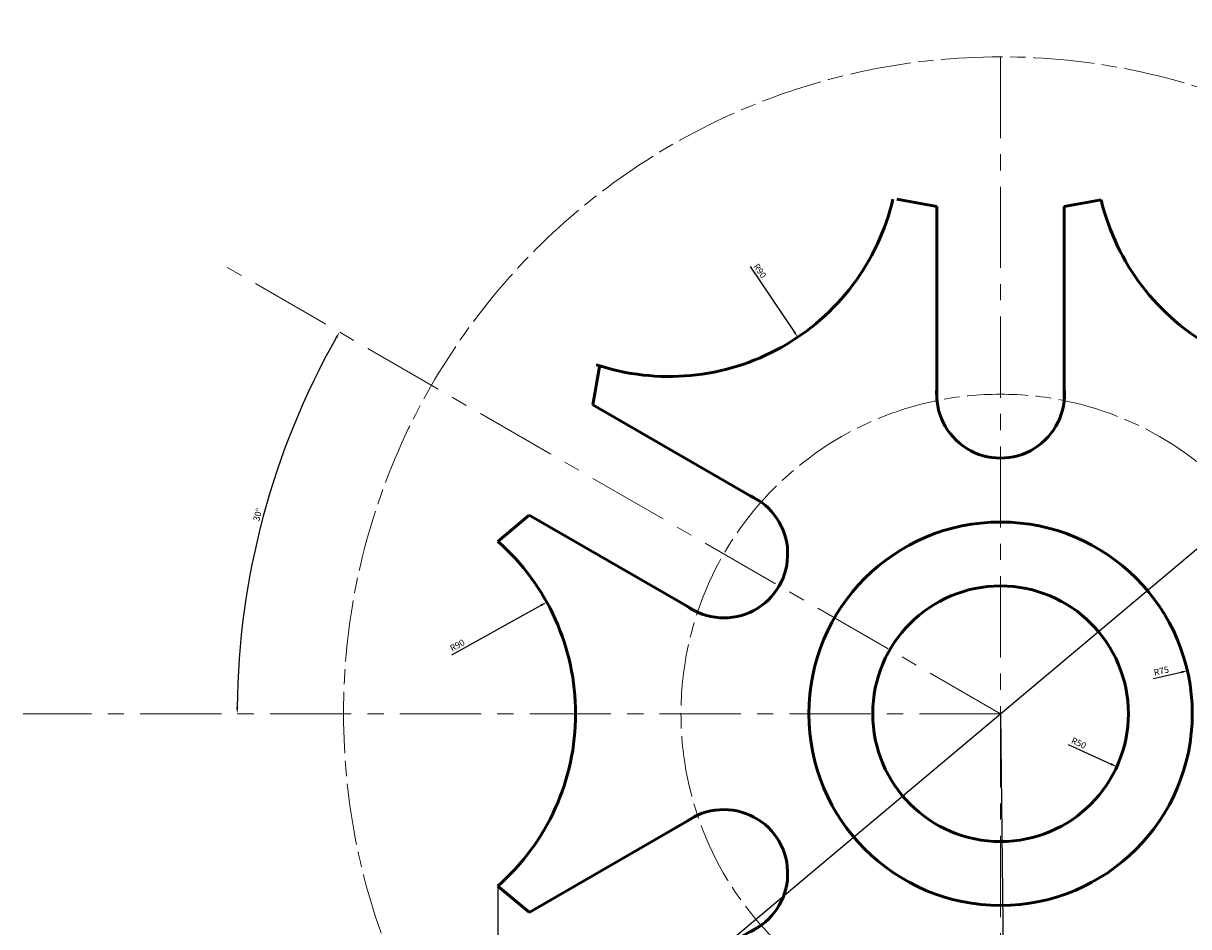
# Model space of a CAD drawing. Units: millimetres. Extents: x 1944 to 2645, y 1235 to 1798.
# Tile 2 of 3: x 1944 to 2400, y 1444 to 1798. Entities that reach past the tile are written whole.
import ezdxf

# ---------------------------------------------------------------- set-up
doc = ezdxf.new("R2010")
doc.units = ezdxf.units.MM
doc.linetypes.add('ACAD_ISO08W100', pattern=[36, 24, -3, 6, -3])
doc.linetypes.add('CENTER', pattern=[50.8, 31.75, -6.35, 6.35, -6.35])
for name, color, linetype, lineweight in [('M-CNTR', 4, 'CENTER', 18), ('M-CONS', 8, 'ACAD_ISO08W100', 18), ('M-DIMS', 2, 'Continuous', 25), ('M-OUTL', 7, 'Continuous', 50)]:
    doc.layers.add(name, color=color, linetype=linetype, lineweight=lineweight)
doc.styles.get("Standard").update_dxf_attribs({"font": 'arial.ttf'})
doc.dimstyles.new('ISO-25', dxfattribs={"dimtxt": 2.5, "dimasz": 2.5, "dimexe": 1.25, "dimexo": 0.625, "dimtad": 1, "dimdec": 1, "dimdsep": 46, "dimtxsty": 'Standard', "dimcen": 2.5, "dimadec": 0, "dimazin": 0, "dimtfac": 1, "dimtdec": 1, "dimtmove": 0, "dimatfit": 3, "dimfxl": 1, "dimarcsym": 0})

# ---------------------------------------------------------------- blocks, each defined once
blk = doc.blocks.new('*D1')
at = {"layer": 'Defpoints', "color": 0, "lineweight": 100, "transparency": 16777216}
for p in [(2023.61, 1702.36), (2045.56, 1629.82), (1943.88, 1527.69), (2326.15, 1527.69), (2326.15, 1527.69)]:
    blk.add_point(p, dxfattribs=at)
at = {"layer": 'M-DIMS', "color": 0, "lineweight": -2, "transparency": 16777216}
blk.add_arc((2326.15, 1527.69), 298.6, 150.4797, 179.5203, dxfattribs=at)
at = {"layer": 'M-DIMS', "color": 0, "lineweight": 100, "transparency": 16777216}
for points in [[(2065.95, 1675.03), (2066.68, 1674.61), (2067.56, 1676.99)], [(2027.98, 1530.19), (2027.15, 1530.19), (2027.55, 1527.69)]]:
    blk.add_solid(points, dxfattribs=at)
at = {"layer": 'M-DIMS', "color": 0, "transparency": 16777216, "insert": (2035.89, 1605.47), "char_height": 2.5, "attachment_point": 5, "rotation": 75}
blk.add_mtext('30°', dxfattribs=at)
blk = doc.blocks.new('*D2')
at = {"layer": 'Defpoints', "color": 0, "lineweight": 100, "transparency": 16777216}
for p in [(2326.15, 1527.69), (2371.65, 1506.95)]:
    blk.add_point(p, dxfattribs=at)
at = {"layer": 'M-DIMS', "color": 0, "lineweight": -2, "transparency": 16777216}
blk.add_line((2352.56, 1515.66), (2369.37, 1507.99), dxfattribs=at)
at = {"layer": 'M-DIMS', "color": 0, "lineweight": 100, "transparency": 16777216}
blk.add_solid([(2369.54, 1508.37), (2369.2, 1507.61), (2371.65, 1506.95)], dxfattribs=at)
at = {"layer": 'M-DIMS', "color": 0, "transparency": 16777216, "insert": (2356.63, 1515.89), "char_height": 2.5, "attachment_point": 5, "rotation": 335.4967}
blk.add_mtext('R50', dxfattribs=at)
blk = doc.blocks.new('*D4')
at = {"layer": 'Defpoints', "color": 0, "lineweight": 100, "transparency": 16777216}
for p in [(2399.25, 1544.48), (2326.15, 1527.69)]:
    blk.add_point(p, dxfattribs=at)
at = {"layer": 'M-DIMS', "color": 0, "lineweight": -2, "transparency": 16777216}
blk.add_line((2386, 1541.43), (2396.81, 1543.92), dxfattribs=at)
at = {"layer": 'M-DIMS', "color": 0, "lineweight": 100, "transparency": 16777216}
blk.add_solid([(2396.72, 1544.32), (2396.9, 1543.51), (2399.25, 1544.48)], dxfattribs=at)
at = {"layer": 'M-DIMS', "color": 0, "transparency": 16777216, "insert": (2389.1, 1544.09), "char_height": 2.5, "attachment_point": 5, "rotation": 12.9324}
blk.add_mtext('R75', dxfattribs=at)
blk = doc.blocks.new('*D6')
at = {"layer": 'Defpoints', "color": 0, "lineweight": 100, "transparency": 16777216}
for p in [(2326.15, 1527.69), (2327.52, 1402.7)]:
    blk.add_point(p, dxfattribs=at)
at = {"layer": 'M-DIMS', "color": 0, "lineweight": -2, "transparency": 16777216}
for p, q in [((2326.15, 1527.69), (2327.52, 1402.7)), ((2327.85, 1372.49), (2327.55, 1400.2))]:
    blk.add_line(p, q, dxfattribs=at)
at = {"layer": 'M-DIMS', "color": 0, "lineweight": 100, "transparency": 16777216}
blk.add_solid([(2327.96, 1400.2), (2327.13, 1400.19), (2327.52, 1402.7)], dxfattribs=at)
at = {"layer": 'M-DIMS', "color": 0, "transparency": 16777216, "insert": (2329.7, 1377.1), "char_height": 2.5, "attachment_point": 5, "rotation": 270.6275}
blk.add_mtext('R125', dxfattribs=at)
blk = doc.blocks.new('*D13')
at = {"layer": 'Defpoints', "color": 0, "lineweight": 100, "transparency": 16777216}
for p in [(2160.02, 1723.78), (2492.28, 1331.61)]:
    blk.add_point(p, dxfattribs=at)
at = {"layer": 'M-DIMS', "color": 0, "lineweight": -2, "transparency": 16777216}
blk.add_line((2467.27, 1361.13), (2490.67, 1333.51), dxfattribs=at)
at = {"layer": 'M-DIMS', "color": 0, "lineweight": 100, "transparency": 16777216}
blk.add_solid([(2490.98, 1333.78), (2490.35, 1333.24), (2492.28, 1331.61)], dxfattribs=at)
at = {"layer": 'M-DIMS', "color": 0, "transparency": 16777216, "insert": (2471.84, 1358.79), "char_height": 2.5, "attachment_point": 5, "rotation": 310.2727}
blk.add_mtext('∅514', dxfattribs=at)
blk = doc.blocks.new('*D14')
at = {"layer": 'Defpoints', "color": 0, "lineweight": 100, "transparency": 16777216}
for p in [(2196.48, 1749.62), (2246.84, 1675.02)]:
    blk.add_point(p, dxfattribs=at)
at = {"layer": 'M-DIMS', "color": 0, "lineweight": -2, "transparency": 16777216}
blk.add_line((2228.16, 1702.69), (2245.44, 1677.1), dxfattribs=at)
at = {"layer": 'M-DIMS', "color": 0, "lineweight": 100, "transparency": 16777216}
blk.add_solid([(2245.78, 1677.33), (2245.09, 1676.86), (2246.84, 1675.02)], dxfattribs=at)
at = {"layer": 'M-DIMS', "color": 0, "transparency": 16777216, "insert": (2231.76, 1700.77), "char_height": 2.5, "attachment_point": 5, "rotation": 304.0183}
blk.add_mtext('R90', dxfattribs=at)
blk = doc.blocks.new('*D15')
at = {"layer": 'Defpoints', "color": 0, "lineweight": 100, "transparency": 16777216}
for p in [(2148.64, 1571.34), (2069.93, 1527.69)]:
    blk.add_point(p, dxfattribs=at)
at = {"layer": 'M-DIMS', "color": 0, "lineweight": -2, "transparency": 16777216}
blk.add_line((2111.56, 1550.78), (2146.45, 1570.13), dxfattribs=at)
at = {"layer": 'M-DIMS', "color": 0, "lineweight": 100, "transparency": 16777216}
blk.add_solid([(2146.25, 1570.49), (2146.66, 1569.77), (2148.64, 1571.34)], dxfattribs=at)
at = {"layer": 'M-DIMS', "color": 0, "transparency": 16777216, "insert": (2113.8, 1554.19), "char_height": 2.5, "attachment_point": 5, "rotation": 29.013}
blk.add_mtext('R90', dxfattribs=at)
blk = doc.blocks.new('GENEVA-RADIAL-SLOT-R25')
for p, q in [((0.13, 76), (0.13, 0)), ((49.87, 76), (49.87, 0))]:
    blk.add_line(p, q)
blk.add_arc((25, 73.5), 25, 354.2608, 185.7392)
blk = doc.blocks.new('*D17')
at = {"layer": 'Defpoints', "color": 0, "lineweight": 100, "transparency": 16777216}
for p in [(2129.55, 1460.27), (2522.75, 1460.27), (2522.75, 1236.69)]:
    blk.add_point(p, dxfattribs=at)
at = {"layer": 'M-DIMS', "color": 0, "lineweight": -2, "transparency": 16777216}
for p, q in [((2129.55, 1459.64), (2129.55, 1235.44)), ((2522.75, 1459.64), (2522.75, 1235.44)), ((2132.05, 1236.69), (2520.25, 1236.69))]:
    blk.add_line(p, q, dxfattribs=at)
at = {"layer": 'M-DIMS', "color": 0, "lineweight": 100, "transparency": 16777216}
for points in [[(2132.05, 1237.11), (2132.05, 1236.27), (2129.55, 1236.69)], [(2520.25, 1237.11), (2520.25, 1236.27), (2522.75, 1236.69)]]:
    blk.add_solid(points, dxfattribs=at)
at = {"layer": 'M-DIMS', "color": 0, "transparency": 16777216, "insert": (2326.15, 1238.59), "char_height": 2.5, "attachment_point": 5}
blk.add_mtext('393.2', dxfattribs=at)
blk = doc.blocks.new('*D18')
at = {"layer": 'Defpoints', "color": 0, "lineweight": 100, "transparency": 16777216}
for p in [(2522.96, 1692.97), (2129.34, 1362.42)]:
    blk.add_point(p, dxfattribs=at)
at = {"layer": 'M-DIMS', "color": 0, "lineweight": -2, "transparency": 16777216}
for p, q in [((2644.67, 1795.18), (2524.87, 1694.57)), ((2129.34, 1362.42), (2522.96, 1692.97)), ((2127.43, 1360.81), (2125.51, 1359.2))]:
    blk.add_line(p, q, dxfattribs=at)
at = {"layer": 'M-DIMS', "color": 0, "lineweight": 100, "transparency": 16777216}
for points in [[(2524.61, 1694.89), (2525.14, 1694.25), (2522.96, 1692.97)], [(2127.16, 1361.13), (2127.69, 1360.49), (2129.34, 1362.42)]]:
    blk.add_solid(points, dxfattribs=at)
at = {"layer": 'M-DIMS', "color": 0, "transparency": 16777216, "insert": (2639.78, 1793.64), "char_height": 2.5, "attachment_point": 5, "rotation": 40.0225}
blk.add_mtext('∅514', dxfattribs=at)

msp = doc.modelspace()

# ---------------------------------------------------------------- linework, layer by layer
at = {"layer": 'M-CNTR'}
for p, q in [((2326.15, 1784.69), (2326.15, 1270.69)), ((2326.15, 1527.69), (2023.61, 1702.36)), ((2326.15, 1527.69), (1943.88, 1527.69))]:
    msp.add_line(p, q, dxfattribs=at)
at = {"layer": 'M-CONS'}
for radius in [257, 125]:
    msp.add_circle((2326.15, 1527.69), radius, dxfattribs=at)
at = {"layer": 'M-OUTL'}
for p, q in [((2301.28, 1726.19), (2285.52, 1728.97)), ((2351.02, 1726.19), (2365.52, 1728.75)), ((2166.68, 1648.48), (2169.46, 1664.24)), ((2141.81, 1605.4), (2129.55, 1595.11)), ((2141.81, 1449.98), (2129.55, 1460.27))]:
    msp.add_line(p, q, dxfattribs=at)
for radius in [75, 50]:
    msp.add_circle((2326.15, 1527.69), radius, dxfattribs=at)
for centre, start, end in [((2196.48, 1749.62), 251.5652, 346.7342), ((2453.06, 1749.62), 193.4116, 289.27), ((2069.93, 1527.69), 311.4834, 48.5166)]:
    msp.add_arc(centre, 90, start, end, dxfattribs=at)

# ---------------------------------------------------------------- block references
for p, rotation in [((2351.15, 1726.19), 180), ((2166.74, 1648.59), 239.9999999999997), ((2141.74, 1450.09), 300.0000000000004)]:
    msp.add_blockref('GENEVA-RADIAL-SLOT-R25', p, dxfattribs=dict(at, rotation=rotation))

# ---------------------------------------------------------------- dimensions: what is measured, and where the dimension line sits
at = {"layer": 'M-DIMS'}
for p1, p2, override, picture, middle in [((2129.34, 1362.42), (2522.96, 1692.97), {"dimdec": 0, "dimlfac": 1, "dimrnd": 0, "dimzin": 0, "dimdsep": 46, "dimlunit": 2}, '*D18', (2641.04, 1792.13)), ((2160.02, 1723.78), (2492.28, 1331.61), {"dimclrd": 0, "dimclre": 0, "dimclrt": 0}, '*D13', (2470.33, 1357.51))]:
    dim = msp.add_diameter_dim_2p(p1=p1, p2=p2, dimstyle='ISO-25', override=override, dxfattribs=at)
    dim.commit()
    dim.dimension.update_dxf_attribs({"geometry": picture, "text_midpoint": middle, "dimtype": 163})
for center, mpoint, picture, middle in [((2196.48, 1749.62), (2246.84, 1675.02), '*D14', (2230.18, 1699.7)), ((2069.93, 1527.69), (2148.64, 1571.34), '*D15', (2114.72, 1552.53)), ((2326.15, 1527.69), (2399.25, 1544.48), '*D4', (2389.53, 1542.24)), ((2326.15, 1527.69), (2371.65, 1506.95), '*D2', (2355.84, 1514.16)), ((2326.15, 1527.69), (2327.52, 1402.7), '*D6', (2327.8, 1377.08))]:
    dim = msp.add_radius_dim(center=center, mpoint=mpoint, dimstyle='ISO-25', override={"dimclrd": 0, "dimclre": 0, "dimclrt": 0}, dxfattribs=at)
    dim.commit()
    dim.dimension.update_dxf_attribs({"geometry": picture, "text_midpoint": middle, "dimtype": 164})
dim = msp.add_angular_dim_2l(base=(2045.56, 1629.82), line1=((2326.15, 1527.69), (2023.61, 1702.36)), line2=((2326.15, 1527.69), (1943.88, 1527.69)), dimstyle='ISO-25', override={"dimclrd": 0, "dimclre": 0, "dimclrt": 0}, dxfattribs=at)
dim.commit()
dim.dimension.update_dxf_attribs({"geometry": '*D1', "text_midpoint": (2035.89, 1605.47)})
dim = msp.add_linear_dim(base=(2522.75, 1236.69), p1=(2129.55, 1460.27), p2=(2522.75, 1460.27), dimstyle='ISO-25', override={"dimdec": 1, "dimlfac": 1, "dimrnd": 0, "dimzin": 0, "dimdsep": 46, "dimlunit": 2}, dxfattribs=at)
dim.commit()
dim.dimension.update_dxf_attribs({"geometry": '*D17', "text_midpoint": (2326.15, 1238.59)})

doc.saveas('drawing.dxf')
